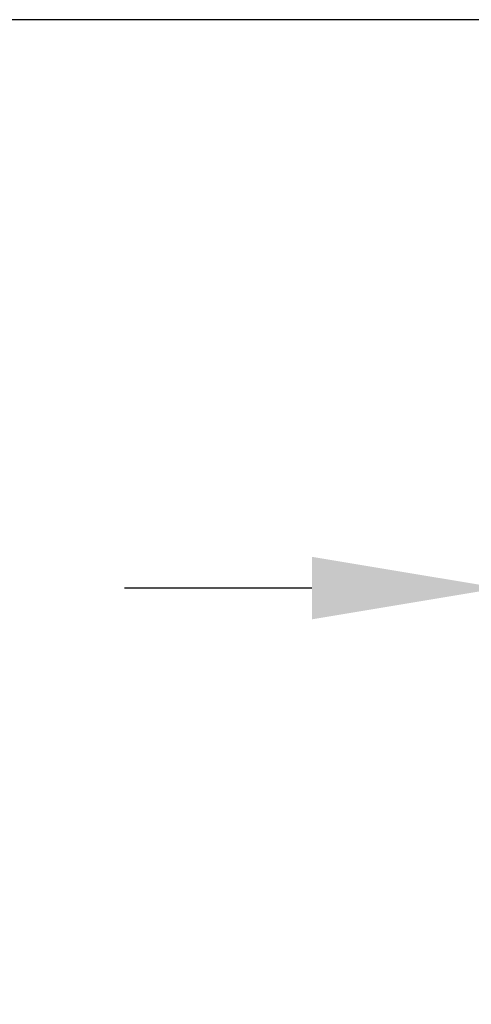
# Model space of a CAD drawing. Units: inches. Extents: x 2091 to 2899, y 967 to 2217.
# Tile 106 of 256: x 2192.88 to 2202.51, y 1131.25 to 1152.25. Entities that reach past the tile are written whole.
import ezdxf

# ---------------------------------------------------------------- set-up
doc = ezdxf.new("R2010")
doc.units = ezdxf.units.IN
doc.layers.add('A-ANNO-DIMS', color=2, linetype='Continuous', lineweight=18)
doc.styles.get("Standard").update_dxf_attribs({"font": 'arial.ttf'})
doc.dimstyles.new('ISO-25', dxfattribs={"dimtxt": 4, "dimasz": 4, "dimexe": 1.25, "dimexo": 0.625, "dimtad": 1, "dimdec": 0, "dimlunit": 3, "dimtxsty": 'Standard', "dimcen": 2.5, "dimadec": 0, "dimazin": 0, "dimtfac": 1, "dimtdec": 0, "dimtmove": 0, "dimatfit": 3, "dimfxl": 1, "dimarcsym": 0})

# ---------------------------------------------------------------- blocks, each defined once
blk = doc.blocks.new('*D37')
at = {"layer": 'A-ANNO-DIMS', "color": 0, "lineweight": -2, "transparency": 16777216}
for p, q in [((2203.116, 1151.622), (2203.116, 1138.874)), ((2212.276, 1151.622), (2212.276, 1138.874)), ((2199.116, 1140.124), (2195.116, 1140.124)), ((2203.116, 1140.124), (2212.276, 1140.124)), ((2216.276, 1140.124), (2245.908, 1140.124))]:
    blk.add_line(p, q, dxfattribs=at)
at = {"layer": 'A-ANNO-DIMS', "color": 0, "transparency": 16777216}
for points in [[(2199.116, 1140.79), (2199.116, 1139.457), (2203.116, 1140.124)], [(2216.276, 1140.79), (2216.276, 1139.457), (2212.276, 1140.124)]]:
    blk.add_solid(points, dxfattribs=at)
at = {"layer": 'Defpoints', "color": 0, "transparency": 16777216}
for p in [(2203.116, 1152.247), (2212.276, 1152.247), (2212.276, 1140.124)]:
    blk.add_point(p, dxfattribs=at)
at = {"layer": 'A-ANNO-DIMS', "color": 0, "transparency": 16777216, "insert": (2233.092, 1142.791), "char_height": 4, "attachment_point": 5}
blk.add_mtext('0\'-9" TYP.', dxfattribs=at)
blk = doc.blocks.new('*D91')
at = {"layer": 'A-ANNO-DIMS', "color": 0, "lineweight": -2, "transparency": 16777216}
for p, q in [((2211.651, 1152.247), (2098.311, 1152.247)), ((2099.561, 1103.919), (2099.561, 1148.247)), ((2211.519, 1099.919), (2098.311, 1099.919))]:
    blk.add_line(p, q, dxfattribs=at)
at = {"layer": 'A-ANNO-DIMS', "color": 0, "transparency": 16777216}
for points in [[(2098.895, 1148.247), (2100.228, 1148.247), (2099.561, 1152.247)], [(2098.895, 1103.919), (2100.228, 1103.919), (2099.561, 1099.919)]]:
    blk.add_solid(points, dxfattribs=at)
at = {"layer": 'Defpoints', "color": 0, "transparency": 16777216}
for p in [(2099.561, 1152.247), (2212.276, 1152.247), (2212.144, 1099.919)]:
    blk.add_point(p, dxfattribs=at)
at = {"layer": 'A-ANNO-DIMS', "color": 0, "transparency": 16777216, "insert": (2096.868, 1126.083), "char_height": 4, "attachment_point": 5, "rotation": 90}
blk.add_mtext('4\'-4 1/2"', dxfattribs=at)

msp = doc.modelspace()

# ---------------------------------------------------------------- dimensions: what is measured, and where the dimension line sits
at = {"layer": 'A-ANNO-DIMS'}
dim = msp.add_linear_dim(base=(2099.561, 1152.247), p1=(2212.144, 1099.919), p2=(2212.276, 1152.247), angle=90, dimstyle='ISO-25', override={"dimdec": 1, "dimlfac": 1, "dimrnd": 0, "dimzin": 1, "dimdsep": 46, "dimlunit": 4, "dimfrac": 2}, dxfattribs=at)
dim.commit()
dim.dimension.update_dxf_attribs({"geometry": '*D91', "text_midpoint": (2096.868, 1126.083)})
dim = msp.add_linear_dim(base=(2212.276, 1140.124), p1=(2203.116, 1152.247), p2=(2212.276, 1152.247), text='<> TYP.', dimstyle='ISO-25', override={"dimdec": 1, "dimlfac": 1, "dimrnd": 0, "dimzin": 1, "dimdsep": 46, "dimlunit": 4, "dimfrac": 2}, dxfattribs=at)
dim.commit()
dim.dimension.update_dxf_attribs({"geometry": '*D37', "text_midpoint": (2233.092, 1142.791)})

doc.saveas('drawing.dxf')
